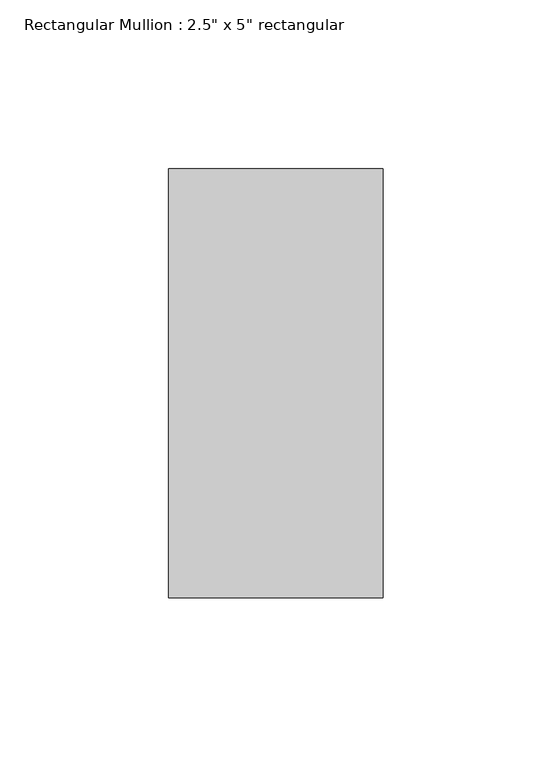
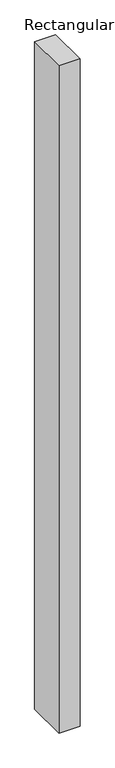
"""IFC4 building model written with IfcOpenShell, lengths in millimetres: member geometry."""

from ifc_helpers import new_model, si_unit, frame, origin, place, context, project, spatial, polyline, outline, extrude, source, transform, mapped, element, save


def member_7cbddb58(model_context):
    return source(origin(), model_context, "Body", "SweptSolid", [
        extrude(outline(polyline([(31.75, 63.5), (31.75, -63.5), (-31.75, -63.5), (-31.75, 63.5), (31.75, 63.5)])), frame((0.0, 0.0, -2133.6), z_axis=(0.0, 0.0, 1.0), x_axis=(1.0, 0.0, 0.0)), (0.0, 0.0, 1.0), 2133.6),
    ])


if __name__ == "__main__":
    model = new_model("IFC4")
    model_context = context("Model", 3, world=origin())
    ifc_project = project(units=[si_unit("LENGTHUNIT", "METRE", prefix="MILLI")], contexts=[model_context])
    site = spatial("IfcSite", under=ifc_project)
    building = spatial("IfcBuilding", under=site)
    placement = place(None, origin())
    member_shape = member_7cbddb58(model_context)
    element("IfcMember", 1, ObjectType="Rectangular Mullion : 2.5\" x 5\" rectangular", at=placement, inside=building, context=model_context, shape_type="MappedRepresentation", body=[
        mapped(member_shape, transform((0.0, 0.0, 0.0), x_axis=(1.0, 0.0, 0.0), y_axis=(0.0, 1.0, 0.0), z_axis=(0.0, 0.0, 1.0))),
    ])
    save(model, "model.ifc")

# Revit data of these elements
# Type "Rectangular Mullion : 2.5\" x 5\" rectangular"
#   built-in parameter 1007304 = 0.416667 (stored number, unit not read)
#   built-in parameter 1007301 = 0.104167 (stored number, unit not read)
#   built-in parameter 1007300 = 0.104167 (stored number, unit not read)
# Element 1 (IfcMember, "Rectangular Mullion : 2.5\" x 5\" rectangular")
#   Materials on its faces: "door black"
# Materials
#   "door black": class "Generic", colour RGB 120 120 120, transparency 0, Cost = 0
